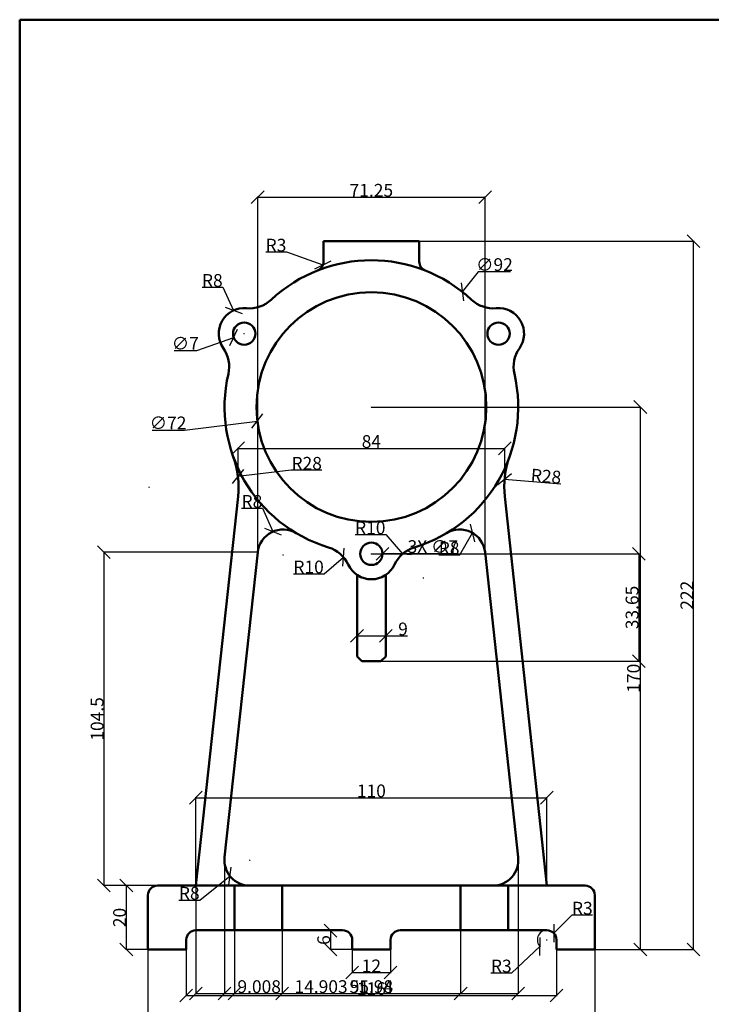
# Model space of a CAD drawing. Units: millimetres. Extents: x -13 to 343, y 323 to 787.
# Tile 2 of 3: x -13 to 204, y 479 to 787. Entities that reach past the tile are written whole.
import ezdxf

# ---------------------------------------------------------------- set-up
doc = ezdxf.new("R2010")
doc.units = ezdxf.units.MM
doc.header["$MEASUREMENT"] = 0
doc.header["$PDMODE"] = 3
doc.header["$PDSIZE"] = -8
for name, color, linetype, lineweight in [('M-DIMS', 2, 'Continuous', 25), ('M-OUTL', 7, 'Continuous', 50), ('M-TTLB', 7, 'Continuous', 50)]:
    doc.layers.add(name, color=color, linetype=linetype, lineweight=lineweight)
doc.styles.get("Standard").update_dxf_attribs({"font": 'arial.ttf'})
doc.dimstyles.get("Standard").update_dxf_attribs({"dimtxt": 4, "dimasz": 4, "dimexe": 0.18, "dimexo": 0.0625, "dimgap": 0.09, "dimtad": 1, "dimtoh": 1, "dimdec": 0, "dimzin": 0, "dimdsep": 46, "dimtxsty": 'Standard', "dimblk": 'OBLIQUE', "dimcen": 0.09, "dimclre": 251, "dimadec": 0, "dimazin": 0, "dimtfac": 1, "dimtdec": 0, "dimtofl": 0, "dimtmove": 0, "dimatfit": 3, "dimfxl": 1, "dimtolj": 1, "dimtzin": 0, "dimarcsym": 0})

# ---------------------------------------------------------------- blocks, each defined once
blk = doc.blocks.new('_Oblique')
at = {"color": 0, "linetype": 'ByBlock', "lineweight": -2}
blk.add_line((-0.5, -0.5), (0.5, 0.5), dxfattribs=at)
blk = doc.blocks.new('*D4')
at = {"layer": 'Defpoints', "color": 0, "transparency": 16777216}
for p in [(79.05, 711.47), (81.88, 710.47)]:
    blk.add_point(p, dxfattribs=at)
at = {"layer": 'M-DIMS', "color": 0, "lineweight": -2, "transparency": 16777216}
for p, q in [((63.95, 714.5), (70.49, 714.5)), ((70.49, 714.5), (81.88, 710.47))]:
    blk.add_line(p, q, dxfattribs=at)
at = {"layer": 'M-DIMS', "color": 0, "lineweight": -2, "transparency": 16777216, "xscale": 4, "yscale": 4, "zscale": 4, "rotation": 340.5270961751787}
blk.add_blockref('_Oblique', (81.88, 710.47), dxfattribs=at)
at = {"layer": 'M-DIMS', "color": 0, "transparency": 16777216, "insert": (67.17, 716.63), "char_height": 4, "attachment_point": 5}
blk.add_mtext('\\A1;R3', dxfattribs=at)
blk = doc.blocks.new('*D5')
at = {"layer": 'Defpoints', "color": 0, "transparency": 16777216}
for p in [(53.88, 696.17), (57.22, 688.9)]:
    blk.add_point(p, dxfattribs=at)
at = {"layer": 'M-DIMS', "color": 0, "lineweight": -2, "transparency": 16777216}
for p, q in [((43.99, 703.43), (50.54, 703.43)), ((50.54, 703.43), (53.88, 696.17)), ((57.13, 688.9), (57.31, 688.9)), ((57.22, 688.81), (57.22, 688.99))]:
    blk.add_line(p, q, dxfattribs=at)
at = {"layer": 'M-DIMS', "color": 0, "lineweight": -2, "transparency": 16777216, "xscale": 4, "yscale": 4, "zscale": 4, "rotation": 294.6792634870832}
blk.add_blockref('_Oblique', (53.88, 696.17), dxfattribs=at)
at = {"layer": 'M-DIMS', "color": 0, "transparency": 16777216, "insert": (47.22, 705.57), "char_height": 4, "attachment_point": 5}
blk.add_mtext('\\A1;R8', dxfattribs=at)
blk = doc.blocks.new('*D6')
at = {"layer": 'Defpoints', "color": 0, "transparency": 16777216}
for p in [(138.77, 643.18), (166.67, 640.82)]:
    blk.add_point(p, dxfattribs=at)
at = {"layer": 'M-DIMS', "color": 0, "lineweight": -2, "transparency": 16777216}
blk.add_line((156.46, 641.69), (138.77, 643.18), dxfattribs=at)
at = {"layer": 'M-DIMS', "color": 0, "lineweight": -2, "transparency": 16777216, "xscale": 4, "yscale": 4, "zscale": 4, "rotation": 175.1553930412952}
blk.add_blockref('_Oblique', (138.77, 643.18), dxfattribs=at)
at = {"layer": 'M-DIMS', "color": 0, "transparency": 16777216, "insert": (151.78, 644.22), "char_height": 4, "attachment_point": 5, "rotation": 355.1554}
blk.add_mtext('\\A1;R28', dxfattribs=at)
blk = doc.blocks.new('*D7')
at = {"layer": 'Defpoints', "color": 0, "transparency": 16777216}
for p in [(88.31, 618.84), (80.72, 612.33)]:
    blk.add_point(p, dxfattribs=at)
at = {"layer": 'M-DIMS', "color": 0, "lineweight": -2, "transparency": 16777216}
for p, q in [((82.24, 613.63), (88.31, 618.84)), ((72.6, 613.63), (82.24, 613.63))]:
    blk.add_line(p, q, dxfattribs=at)
at = {"layer": 'M-DIMS', "color": 0, "lineweight": -2, "transparency": 16777216, "xscale": 4, "yscale": 4, "zscale": 4, "rotation": 40.60279433407489}
blk.add_blockref('_Oblique', (88.31, 618.84), dxfattribs=at)
at = {"layer": 'M-DIMS', "color": 0, "transparency": 16777216, "insert": (77.38, 615.76), "char_height": 4, "attachment_point": 5}
blk.add_mtext('\\A1;R10', dxfattribs=at)
blk = doc.blocks.new('*D8')
at = {"layer": 'Defpoints', "color": 0, "transparency": 16777216}
for p in [(128.77, 626.43), (124.73, 619.53)]:
    blk.add_point(p, dxfattribs=at)
at = {"layer": 'M-DIMS', "color": 0, "lineweight": -2, "transparency": 16777216}
for p, q in [((124.73, 619.53), (128.77, 626.43)), ((118.18, 619.53), (124.73, 619.53))]:
    blk.add_line(p, q, dxfattribs=at)
at = {"layer": 'M-DIMS', "color": 0, "lineweight": -2, "transparency": 16777216, "xscale": 4, "yscale": 4, "zscale": 4, "rotation": 59.62070806572377}
blk.add_blockref('_Oblique', (128.77, 626.43), dxfattribs=at)
at = {"layer": 'M-DIMS', "color": 0, "transparency": 16777216, "insert": (121.41, 621.66), "char_height": 4, "attachment_point": 5}
blk.add_mtext('\\A1;R8', dxfattribs=at)
blk = doc.blocks.new('*D9')
at = {"layer": 'Defpoints', "color": 0, "transparency": 16777216}
for p in [(152.05, 498.9), (149.87, 496.84)]:
    blk.add_point(p, dxfattribs=at)
at = {"layer": 'M-DIMS', "color": 0, "lineweight": -2, "transparency": 16777216}
for p, q in [((151.96, 498.9), (152.14, 498.9)), ((152.05, 498.81), (152.05, 498.99)), ((141.07, 488.55), (149.87, 496.84)), ((134.53, 488.55), (141.07, 488.55))]:
    blk.add_line(p, q, dxfattribs=at)
blk.add_arc((152.05, 498.9), 3, 91.1937, 226.7257, dxfattribs=at)
at = {"layer": 'M-DIMS', "color": 0, "lineweight": -2, "transparency": 16777216, "xscale": 4, "yscale": 4, "zscale": 4, "rotation": 43.28792637846206}
blk.add_blockref('_Oblique', (149.87, 496.84), dxfattribs=at)
at = {"layer": 'M-DIMS', "color": 0, "transparency": 16777216, "insert": (137.76, 490.68), "char_height": 4, "attachment_point": 5}
blk.add_mtext('\\A1;R3', dxfattribs=at)
blk = doc.blocks.new('*D10')
at = {"layer": 'Defpoints', "color": 0, "transparency": 16777216}
for p in [(125.54, 702.01), (68.56, 629.78)]:
    blk.add_point(p, dxfattribs=at)
at = {"layer": 'M-DIMS', "color": 0, "lineweight": -2, "transparency": 16777216}
for p, q in [((130.5, 708.29), (125.54, 702.01)), ((140.63, 708.29), (130.5, 708.29)), ((96.96, 665.9), (97.14, 665.9)), ((97.05, 665.81), (97.05, 665.99))]:
    blk.add_line(p, q, dxfattribs=at)
at = {"layer": 'M-DIMS', "color": 0, "lineweight": -2, "transparency": 16777216, "xscale": 4, "yscale": 4, "zscale": 4, "rotation": 231.7324011261606}
blk.add_blockref('_Oblique', (125.54, 702.01), dxfattribs=at)
at = {"layer": 'M-DIMS', "color": 0, "transparency": 16777216, "insert": (135.61, 710.54), "char_height": 4, "attachment_point": 5}
blk.add_mtext('\\A1;∅92', dxfattribs=at)
blk = doc.blocks.new('*D11')
at = {"layer": 'Defpoints', "color": 0, "transparency": 16777216}
for p in [(132.78, 670.3), (61.32, 661.49)]:
    blk.add_point(p, dxfattribs=at)
at = {"layer": 'M-DIMS', "color": 0, "lineweight": -2, "transparency": 16777216}
for p, q in [((96.96, 665.9), (97.14, 665.9)), ((97.05, 665.81), (97.05, 665.99)), ((38.45, 658.68), (61.32, 661.49)), ((28.32, 658.68), (38.45, 658.68))]:
    blk.add_line(p, q, dxfattribs=at)
at = {"layer": 'M-DIMS', "color": 0, "lineweight": -2, "transparency": 16777216, "xscale": 4, "yscale": 4, "zscale": 4, "rotation": 7.023598730046072}
blk.add_blockref('_Oblique', (61.32, 661.49), dxfattribs=at)
at = {"layer": 'M-DIMS', "color": 0, "transparency": 16777216, "insert": (33.34, 660.92), "char_height": 4, "attachment_point": 5}
blk.add_mtext('\\A1;∅72', dxfattribs=at)
blk = doc.blocks.new('*D12')
at = {"layer": 'Defpoints', "color": 0, "transparency": 16777216}
for p in [(60.51, 690.07), (53.92, 687.72)]:
    blk.add_point(p, dxfattribs=at)
at = {"layer": 'M-DIMS', "color": 0, "lineweight": -2, "transparency": 16777216}
for p, q in [((57.13, 688.9), (57.31, 688.9)), ((57.22, 688.81), (57.22, 688.99)), ((42.33, 683.58), (53.92, 687.72)), ((35.26, 683.58), (42.33, 683.58))]:
    blk.add_line(p, q, dxfattribs=at)
at = {"layer": 'M-DIMS', "color": 0, "lineweight": -2, "transparency": 16777216, "xscale": 4, "yscale": 4, "zscale": 4, "rotation": 19.63186523037221}
blk.add_blockref('_Oblique', (53.92, 687.72), dxfattribs=at)
at = {"layer": 'M-DIMS', "color": 0, "transparency": 16777216, "insert": (38.75, 685.83), "char_height": 4, "attachment_point": 5}
blk.add_mtext('\\A1;∅7', dxfattribs=at)
blk = doc.blocks.new('*D13')
at = {"layer": 'Defpoints', "color": 0, "transparency": 16777216}
for p in [(97.14, 665.9), (167.05, 495.9), (181.31, 495.9)]:
    blk.add_point(p, dxfattribs=at)
at = {"layer": 'M-DIMS', "color": 0, "lineweight": -2, "transparency": 16777216}
for p, q in [((97.21, 665.9), (181.49, 665.9)), ((181.31, 665.9), (181.31, 495.9)), ((167.12, 495.9), (181.49, 495.9))]:
    blk.add_line(p, q, dxfattribs=at)
at = {"layer": 'M-DIMS', "color": 0, "lineweight": -2, "transparency": 16777216, "xscale": 4, "yscale": 4, "zscale": 4}
for p, rotation in [((181.31, 665.9), 90), ((181.31, 495.9), 270)]:
    blk.add_blockref('_Oblique', p, dxfattribs=dict(at, rotation=rotation))
at = {"layer": 'M-DIMS', "color": 0, "transparency": 16777216, "insert": (179.18, 580.9), "char_height": 4, "attachment_point": 5, "rotation": 90}
blk.add_mtext('\\A1;170', dxfattribs=at)
blk = doc.blocks.new('*D14')
at = {"layer": 'Defpoints', "color": 0, "transparency": 16777216}
for p in [(112.05, 717.9), (198, 717.9), (167.05, 495.9)]:
    blk.add_point(p, dxfattribs=at)
at = {"layer": 'M-DIMS', "color": 0, "lineweight": -2, "transparency": 16777216}
for p, q in [((112.12, 717.9), (198.18, 717.9)), ((198, 495.9), (198, 717.9)), ((167.12, 495.9), (198.18, 495.9))]:
    blk.add_line(p, q, dxfattribs=at)
at = {"layer": 'M-DIMS', "color": 0, "lineweight": -2, "transparency": 16777216, "xscale": 4, "yscale": 4, "zscale": 4}
for p, rotation in [((198, 717.9), 90), ((198, 495.9), 270)]:
    blk.add_blockref('_Oblique', p, dxfattribs=dict(at, rotation=rotation))
at = {"layer": 'M-DIMS', "color": 0, "transparency": 16777216, "insert": (195.9, 606.9), "char_height": 4, "attachment_point": 5, "rotation": 90}
blk.add_mtext('\\A1;222', dxfattribs=at)
blk = doc.blocks.new('*D15')
at = {"layer": 'Defpoints', "color": 0, "transparency": 16777216}
for p in [(27.05, 495.9), (167.05, 495.9), (167.05, 471.86)]:
    blk.add_point(p, dxfattribs=at)
at = {"layer": 'M-DIMS', "color": 0, "lineweight": -2, "transparency": 16777216}
for p, q in [((27.05, 495.83), (27.05, 471.68)), ((167.05, 495.83), (167.05, 471.68)), ((27.05, 471.86), (167.05, 471.86))]:
    blk.add_line(p, q, dxfattribs=at)
at = {"layer": 'M-DIMS', "color": 0, "lineweight": -2, "transparency": 16777216, "xscale": 4, "yscale": 4, "zscale": 4, "rotation": 180}
blk.add_blockref('_Oblique', (27.05, 471.86), dxfattribs=at)
at = {"layer": 'M-DIMS', "color": 0, "lineweight": -2, "transparency": 16777216, "xscale": 4, "yscale": 4, "zscale": 4}
blk.add_blockref('_Oblique', (167.05, 471.86), dxfattribs=at)
at = {"layer": 'M-DIMS', "color": 0, "transparency": 16777216, "insert": (97.05, 473.99), "char_height": 4, "attachment_point": 5}
blk.add_mtext('\\A1;140', dxfattribs=at)
blk = doc.blocks.new('*D16')
at = {"layer": 'Defpoints', "color": 0, "transparency": 16777216}
for p in [(39.05, 495.9), (155.05, 495.9), (155.05, 481.47)]:
    blk.add_point(p, dxfattribs=at)
at = {"layer": 'M-DIMS', "color": 0, "lineweight": -2, "transparency": 16777216}
for p, q in [((39.05, 495.83), (39.05, 481.29)), ((155.05, 495.83), (155.05, 481.29)), ((39.05, 481.47), (155.05, 481.47))]:
    blk.add_line(p, q, dxfattribs=at)
at = {"layer": 'M-DIMS', "color": 0, "lineweight": -2, "transparency": 16777216, "xscale": 4, "yscale": 4, "zscale": 4, "rotation": 180}
blk.add_blockref('_Oblique', (39.05, 481.47), dxfattribs=at)
at = {"layer": 'M-DIMS', "color": 0, "lineweight": -2, "transparency": 16777216, "xscale": 4, "yscale": 4, "zscale": 4}
blk.add_blockref('_Oblique', (155.05, 481.47), dxfattribs=at)
at = {"layer": 'M-DIMS', "color": 0, "transparency": 16777216, "insert": (97.05, 483.6), "char_height": 4, "attachment_point": 5}
blk.add_mtext('\\A1;116', dxfattribs=at)
blk = doc.blocks.new('*D17')
at = {"layer": 'Defpoints', "color": 0, "transparency": 16777216}
for p in [(88.96, 501.76), (84.26, 495.9), (91.05, 495.9)]:
    blk.add_point(p, dxfattribs=at)
at = {"layer": 'M-DIMS', "color": 0, "lineweight": -2, "transparency": 16777216}
for p, q in [((88.9, 501.76), (84.08, 501.76)), ((84.26, 501.76), (84.26, 495.9)), ((90.99, 495.9), (84.08, 495.9))]:
    blk.add_line(p, q, dxfattribs=at)
at = {"layer": 'M-DIMS', "color": 0, "lineweight": -2, "transparency": 16777216, "xscale": 4, "yscale": 4, "zscale": 4}
for p, rotation in [((84.26, 501.76), 90), ((84.26, 495.9), 270)]:
    blk.add_blockref('_Oblique', p, dxfattribs=dict(at, rotation=rotation))
at = {"layer": 'M-DIMS', "color": 0, "transparency": 16777216, "insert": (82.12, 498.83), "char_height": 4, "attachment_point": 5, "rotation": 90}
blk.add_mtext('\\A1;6', dxfattribs=at)
blk = doc.blocks.new('*D18')
at = {"layer": 'Defpoints', "color": 0, "transparency": 16777216}
for p in [(91.05, 495.9), (103.05, 495.9), (103.05, 488.62)]:
    blk.add_point(p, dxfattribs=at)
at = {"layer": 'M-DIMS', "color": 0, "lineweight": -2, "transparency": 16777216}
for p, q in [((91.05, 495.83), (91.05, 488.44)), ((103.05, 495.83), (103.05, 488.44)), ((91.05, 488.62), (103.05, 488.62))]:
    blk.add_line(p, q, dxfattribs=at)
at = {"layer": 'M-DIMS', "color": 0, "lineweight": -2, "transparency": 16777216, "xscale": 4, "yscale": 4, "zscale": 4, "rotation": 180}
blk.add_blockref('_Oblique', (91.05, 488.62), dxfattribs=at)
at = {"layer": 'M-DIMS', "color": 0, "lineweight": -2, "transparency": 16777216, "xscale": 4, "yscale": 4, "zscale": 4}
blk.add_blockref('_Oblique', (103.05, 488.62), dxfattribs=at)
at = {"layer": 'M-DIMS', "color": 0, "transparency": 16777216, "insert": (97.05, 490.72), "char_height": 4, "attachment_point": 5}
blk.add_mtext('\\A1;12', dxfattribs=at)
blk = doc.blocks.new('*D19')
at = {"layer": 'Defpoints', "color": 0, "transparency": 16777216}
for p in [(20.28, 515.9), (33.13, 515.9), (27.05, 495.9)]:
    blk.add_point(p, dxfattribs=at)
at = {"layer": 'M-DIMS', "color": 0, "lineweight": -2, "transparency": 16777216}
for p, q in [((33.07, 515.9), (20.1, 515.9)), ((20.28, 495.9), (20.28, 515.9)), ((26.99, 495.9), (20.1, 495.9))]:
    blk.add_line(p, q, dxfattribs=at)
at = {"layer": 'M-DIMS', "color": 0, "lineweight": -2, "transparency": 16777216, "xscale": 4, "yscale": 4, "zscale": 4}
for p, rotation in [((20.28, 515.9), 90), ((20.28, 495.9), 270)]:
    blk.add_blockref('_Oblique', p, dxfattribs=dict(at, rotation=rotation))
at = {"layer": 'M-DIMS', "color": 0, "transparency": 16777216, "insert": (18.15, 505.9), "char_height": 4, "attachment_point": 5, "rotation": 90}
blk.add_mtext('\\A1;20', dxfattribs=at)
blk = doc.blocks.new('*D20')
at = {"layer": 'Defpoints', "color": 0, "transparency": 16777216}
for p in [(152.05, 543.45), (42.05, 515.9), (152.05, 515.9)]:
    blk.add_point(p, dxfattribs=at)
at = {"layer": 'M-DIMS', "color": 0, "lineweight": -2, "transparency": 16777216}
for p, q in [((42.05, 515.96), (42.05, 543.63)), ((42.05, 543.45), (152.05, 543.45)), ((152.05, 515.96), (152.05, 543.63))]:
    blk.add_line(p, q, dxfattribs=at)
at = {"layer": 'M-DIMS', "color": 0, "lineweight": -2, "transparency": 16777216, "xscale": 4, "yscale": 4, "zscale": 4, "rotation": 180}
blk.add_blockref('_Oblique', (42.05, 543.45), dxfattribs=at)
at = {"layer": 'M-DIMS', "color": 0, "lineweight": -2, "transparency": 16777216, "xscale": 4, "yscale": 4, "zscale": 4}
blk.add_blockref('_Oblique', (152.05, 543.45), dxfattribs=at)
at = {"layer": 'M-DIMS', "color": 0, "transparency": 16777216, "insert": (97.05, 545.58), "char_height": 4, "attachment_point": 5}
blk.add_mtext('\\A1;110', dxfattribs=at)
blk = doc.blocks.new('*D21')
at = {"layer": 'Defpoints', "color": 0, "transparency": 16777216}
for p in [(138.84, 652.95), (55.27, 637.8), (138.84, 637.8)]:
    blk.add_point(p, dxfattribs=at)
at = {"layer": 'M-DIMS', "color": 0, "lineweight": -2, "transparency": 16777216}
for p, q in [((55.27, 637.86), (55.27, 653.13)), ((55.27, 652.95), (138.84, 652.95)), ((138.84, 637.86), (138.84, 653.13))]:
    blk.add_line(p, q, dxfattribs=at)
at = {"layer": 'M-DIMS', "color": 0, "lineweight": -2, "transparency": 16777216, "xscale": 4, "yscale": 4, "zscale": 4, "rotation": 180}
blk.add_blockref('_Oblique', (55.27, 652.95), dxfattribs=at)
at = {"layer": 'M-DIMS', "color": 0, "lineweight": -2, "transparency": 16777216, "xscale": 4, "yscale": 4, "zscale": 4}
blk.add_blockref('_Oblique', (138.84, 652.95), dxfattribs=at)
at = {"layer": 'M-DIMS', "color": 0, "transparency": 16777216, "insert": (97.05, 655.08), "char_height": 4, "attachment_point": 5}
blk.add_mtext('\\A1;84', dxfattribs=at)
blk = doc.blocks.new('*D22')
at = {"layer": 'Defpoints', "color": 0, "transparency": 16777216}
for p in [(101.55, 594.2), (92.55, 591.73), (101.55, 591.73)]:
    blk.add_point(p, dxfattribs=at)
at = {"layer": 'M-DIMS', "color": 0, "lineweight": -2, "transparency": 16777216}
for p, q in [((92.55, 591.79), (92.55, 594.38)), ((92.55, 594.2), (101.55, 594.2)), ((101.55, 591.79), (101.55, 594.38)), ((101.55, 594.2), (108.36, 594.2))]:
    blk.add_line(p, q, dxfattribs=at)
at = {"layer": 'M-DIMS', "color": 0, "lineweight": -2, "transparency": 16777216, "xscale": 4, "yscale": 4, "zscale": 4, "rotation": 180}
blk.add_blockref('_Oblique', (92.55, 594.2), dxfattribs=at)
at = {"layer": 'M-DIMS', "color": 0, "lineweight": -2, "transparency": 16777216, "xscale": 4, "yscale": 4, "zscale": 4}
blk.add_blockref('_Oblique', (101.55, 594.2), dxfattribs=at)
at = {"layer": 'M-DIMS', "color": 0, "transparency": 16777216, "insert": (106.96, 596.33), "char_height": 4, "attachment_point": 5}
blk.add_mtext('\\A1;9', dxfattribs=at)
blk = doc.blocks.new('*D38')
at = {"layer": 'Defpoints', "color": 0, "transparency": 16777216}
for p in [(97.05, 619.9), (94.05, 586.24), (180.85, 586.24)]:
    blk.add_point(p, dxfattribs=at)
at = {"layer": 'M-DIMS', "color": 251, "lineweight": -2, "transparency": 16777216}
for p, q in [((97.12, 619.9), (181.03, 619.9)), ((94.12, 586.24), (181.03, 586.24))]:
    blk.add_line(p, q, dxfattribs=at)
at = {"layer": 'M-DIMS', "color": 0, "lineweight": -2, "transparency": 16777216}
blk.add_line((180.85, 619.9), (180.85, 586.24), dxfattribs=at)
at = {"layer": 'M-DIMS', "color": 0, "lineweight": -2, "transparency": 16777216, "xscale": 4, "yscale": 4, "zscale": 4}
for p, rotation in [((180.85, 619.9), 90), ((180.85, 586.24), 270)]:
    blk.add_blockref('_Oblique', p, dxfattribs=dict(at, rotation=rotation))
at = {"layer": 'M-DIMS', "color": 0, "transparency": 16777216, "insert": (178.72, 603.07), "char_height": 4, "attachment_point": 5, "rotation": 90}
blk.add_mtext('\\A1;33.65', dxfattribs=at)
blk = doc.blocks.new('*D39')
at = {"layer": 'Defpoints', "color": 0, "transparency": 16777216}
for p in [(132.68, 731.7), (61.43, 620.39), (132.68, 620.39)]:
    blk.add_point(p, dxfattribs=at)
at = {"layer": 'M-DIMS', "color": 251, "lineweight": -2, "transparency": 16777216}
for p, q in [((61.43, 620.45), (61.43, 731.88)), ((132.68, 620.45), (132.68, 731.88))]:
    blk.add_line(p, q, dxfattribs=at)
at = {"layer": 'M-DIMS', "color": 0, "lineweight": -2, "transparency": 16777216}
blk.add_line((61.43, 731.7), (132.68, 731.7), dxfattribs=at)
at = {"layer": 'M-DIMS', "color": 0, "lineweight": -2, "transparency": 16777216, "xscale": 4, "yscale": 4, "zscale": 4, "rotation": 180}
blk.add_blockref('_Oblique', (61.43, 731.7), dxfattribs=at)
at = {"layer": 'M-DIMS', "color": 0, "lineweight": -2, "transparency": 16777216, "xscale": 4, "yscale": 4, "zscale": 4}
blk.add_blockref('_Oblique', (132.68, 731.7), dxfattribs=at)
at = {"layer": 'M-DIMS', "color": 0, "transparency": 16777216, "insert": (97.05, 733.83), "char_height": 4, "attachment_point": 5}
blk.add_mtext('\\A1;71.25', dxfattribs=at)
blk = doc.blocks.new('*D40')
at = {"layer": 'Defpoints', "color": 0, "transparency": 16777216}
for p in [(51.06, 524.76), (143.05, 524.76), (143.05, 482.1)]:
    blk.add_point(p, dxfattribs=at)
at = {"layer": 'M-DIMS', "color": 251, "lineweight": -2, "transparency": 16777216}
for p, q in [((51.06, 524.7), (51.06, 481.92)), ((143.05, 524.7), (143.05, 481.92))]:
    blk.add_line(p, q, dxfattribs=at)
at = {"layer": 'M-DIMS', "color": 0, "lineweight": -2, "transparency": 16777216}
blk.add_line((51.06, 482.1), (143.05, 482.1), dxfattribs=at)
at = {"layer": 'M-DIMS', "color": 0, "lineweight": -2, "transparency": 16777216, "xscale": 4, "yscale": 4, "zscale": 4, "rotation": 180}
blk.add_blockref('_Oblique', (51.06, 482.1), dxfattribs=at)
at = {"layer": 'M-DIMS', "color": 0, "lineweight": -2, "transparency": 16777216, "xscale": 4, "yscale": 4, "zscale": 4}
blk.add_blockref('_Oblique', (143.05, 482.1), dxfattribs=at)
at = {"layer": 'M-DIMS', "color": 0, "transparency": 16777216, "insert": (97.05, 484.23), "char_height": 4, "attachment_point": 5}
blk.add_mtext('\\A1;91.98', dxfattribs=at)
blk = doc.blocks.new('*D41')
at = {"layer": 'Defpoints', "color": 0, "transparency": 16777216}
for p in [(51.06, 524.76), (42.05, 515.9), (51.06, 482.1)]:
    blk.add_point(p, dxfattribs=at)
at = {"layer": 'M-DIMS', "color": 251, "lineweight": -2, "transparency": 16777216}
for p, q in [((51.06, 524.7), (51.06, 481.92)), ((42.05, 515.83), (42.05, 481.92))]:
    blk.add_line(p, q, dxfattribs=at)
at = {"layer": 'M-DIMS', "color": 0, "lineweight": -2, "transparency": 16777216}
for p, q in [((42.05, 482.1), (51.06, 482.1)), ((51.06, 482.1), (68.75, 482.1))]:
    blk.add_line(p, q, dxfattribs=at)
at = {"layer": 'M-DIMS', "color": 0, "lineweight": -2, "transparency": 16777216, "xscale": 4, "yscale": 4, "zscale": 4, "rotation": 180}
blk.add_blockref('_Oblique', (42.05, 482.1), dxfattribs=at)
at = {"layer": 'M-DIMS', "color": 0, "lineweight": -2, "transparency": 16777216, "xscale": 4, "yscale": 4, "zscale": 4}
blk.add_blockref('_Oblique', (51.06, 482.1), dxfattribs=at)
at = {"layer": 'M-DIMS', "color": 0, "transparency": 16777216, "insert": (61.9, 484.23), "char_height": 4, "attachment_point": 5}
blk.add_mtext('\\A1;9.008', dxfattribs=at)
blk = doc.blocks.new('*D42')
at = {"layer": 'Defpoints', "color": 0, "transparency": 16777216}
for p in [(61.43, 620.39), (13.25, 515.9), (59.01, 515.9)]:
    blk.add_point(p, dxfattribs=at)
at = {"layer": 'M-DIMS', "color": 251, "lineweight": -2, "transparency": 16777216}
for p, q in [((61.36, 620.39), (13.07, 620.39)), ((58.95, 515.9), (13.07, 515.9))]:
    blk.add_line(p, q, dxfattribs=at)
at = {"layer": 'M-DIMS', "color": 0, "lineweight": -2, "transparency": 16777216}
blk.add_line((13.25, 620.39), (13.25, 515.9), dxfattribs=at)
at = {"layer": 'M-DIMS', "color": 0, "lineweight": -2, "transparency": 16777216, "xscale": 4, "yscale": 4, "zscale": 4}
for p, rotation in [((13.25, 620.39), 90), ((13.25, 515.9), 270)]:
    blk.add_blockref('_Oblique', p, dxfattribs=dict(at, rotation=rotation))
at = {"layer": 'M-DIMS', "color": 0, "transparency": 16777216, "insert": (11.12, 568.14), "char_height": 4, "attachment_point": 5, "rotation": 90}
blk.add_mtext('\\A1;104.5', dxfattribs=at)
blk = doc.blocks.new('*D43')
at = {"layer": 'Defpoints', "color": 0, "transparency": 16777216}
for p in [(54.18, 515.9), (69.08, 515.9), (69.08, 482.1)]:
    blk.add_point(p, dxfattribs=at)
at = {"layer": 'M-DIMS', "color": 251, "lineweight": -2, "transparency": 16777216}
for p, q in [((54.18, 515.83), (54.18, 481.92)), ((69.08, 515.83), (69.08, 481.92))]:
    blk.add_line(p, q, dxfattribs=at)
at = {"layer": 'M-DIMS', "color": 0, "lineweight": -2, "transparency": 16777216}
for p, q in [((54.18, 482.1), (69.08, 482.1)), ((69.08, 482.1), (89.49, 482.1))]:
    blk.add_line(p, q, dxfattribs=at)
at = {"layer": 'M-DIMS', "color": 0, "lineweight": -2, "transparency": 16777216, "xscale": 4, "yscale": 4, "zscale": 4, "rotation": 180}
blk.add_blockref('_Oblique', (54.18, 482.1), dxfattribs=at)
at = {"layer": 'M-DIMS', "color": 0, "lineweight": -2, "transparency": 16777216, "xscale": 4, "yscale": 4, "zscale": 4}
blk.add_blockref('_Oblique', (69.08, 482.1), dxfattribs=at)
at = {"layer": 'M-DIMS', "color": 0, "transparency": 16777216, "insert": (81.29, 484.23), "char_height": 4, "attachment_point": 5}
blk.add_mtext('\\A1;14.903', dxfattribs=at)
blk = doc.blocks.new('*D44')
at = {"layer": 'Defpoints', "color": 0, "transparency": 16777216}
for p in [(69.08, 515.9), (125.02, 515.9), (125.02, 482.1)]:
    blk.add_point(p, dxfattribs=at)
at = {"layer": 'M-DIMS', "color": 251, "lineweight": -2, "transparency": 16777216}
for p, q in [((69.08, 515.83), (69.08, 481.92)), ((125.02, 515.83), (125.02, 481.92))]:
    blk.add_line(p, q, dxfattribs=at)
at = {"layer": 'M-DIMS', "color": 0, "lineweight": -2, "transparency": 16777216}
blk.add_line((69.08, 482.1), (125.02, 482.1), dxfattribs=at)
at = {"layer": 'M-DIMS', "color": 0, "lineweight": -2, "transparency": 16777216, "xscale": 4, "yscale": 4, "zscale": 4, "rotation": 180}
blk.add_blockref('_Oblique', (69.08, 482.1), dxfattribs=at)
at = {"layer": 'M-DIMS', "color": 0, "lineweight": -2, "transparency": 16777216, "xscale": 4, "yscale": 4, "zscale": 4}
blk.add_blockref('_Oblique', (125.02, 482.1), dxfattribs=at)
at = {"layer": 'M-DIMS', "color": 0, "transparency": 16777216, "insert": (97.05, 484.23), "char_height": 4, "attachment_point": 5}
blk.add_mtext('\\A1;55.94', dxfattribs=at)
blk = doc.blocks.new('*D65')
at = {"layer": 'Defpoints', "color": 0, "transparency": 16777216}
for p in [(93.55, 619.89), (100.55, 619.9)]:
    blk.add_point(p, dxfattribs=at)
at = {"layer": 'M-DIMS', "color": 251, "lineweight": -2, "transparency": 16777216}
for p, q in [((96.96, 619.9), (97.14, 619.9)), ((97.05, 619.81), (97.05, 619.99))]:
    blk.add_line(p, q, dxfattribs=at)
at = {"layer": 'M-DIMS', "color": 0, "lineweight": -2, "transparency": 16777216}
for p, q in [((108.55, 619.91), (100.55, 619.9)), ((124, 619.91), (108.55, 619.91))]:
    blk.add_line(p, q, dxfattribs=at)
at = {"layer": 'M-DIMS', "color": 0, "lineweight": -2, "transparency": 16777216, "xscale": 4, "yscale": 4, "zscale": 4, "rotation": 180.0631563297542}
blk.add_blockref('_Oblique', (100.55, 619.9), dxfattribs=at)
at = {"layer": 'M-DIMS', "color": 0, "transparency": 16777216, "insert": (116.32, 622.15), "char_height": 4, "attachment_point": 5}
blk.add_mtext('\\A1;3X ∅7', dxfattribs=at)
blk = doc.blocks.new('*D66')
at = {"layer": 'Defpoints', "color": 0, "transparency": 16777216}
for p in [(55.23, 644.14), (27.43, 640.82)]:
    blk.add_point(p, dxfattribs=at)
at = {"layer": 'M-DIMS', "color": 0, "lineweight": -2, "transparency": 16777216}
for p, q in [((71.92, 646.13), (55.23, 644.14)), ((81.57, 646.13), (71.92, 646.13))]:
    blk.add_line(p, q, dxfattribs=at)
at = {"layer": 'M-DIMS', "color": 251, "lineweight": -2, "transparency": 16777216}
for p, q in [((27.34, 640.82), (27.52, 640.82)), ((27.43, 640.73), (27.43, 640.91))]:
    blk.add_line(p, q, dxfattribs=at)
at = {"layer": 'M-DIMS', "color": 0, "lineweight": -2, "transparency": 16777216, "xscale": 4, "yscale": 4, "zscale": 4, "rotation": 186.8108270128715}
blk.add_blockref('_Oblique', (55.23, 644.14), dxfattribs=at)
at = {"layer": 'M-DIMS', "color": 0, "transparency": 16777216, "insert": (76.79, 648.26), "char_height": 4, "attachment_point": 5}
blk.add_mtext('\\A1;R28', dxfattribs=at)
blk = doc.blocks.new('*D67')
at = {"layer": 'Defpoints', "color": 0, "transparency": 16777216}
for p in [(106.82, 619.87), (113.39, 612.33)]:
    blk.add_point(p, dxfattribs=at)
at = {"layer": 'M-DIMS', "color": 0, "lineweight": -2, "transparency": 16777216}
for p, q in [((91.93, 625.91), (101.57, 625.91)), ((101.57, 625.91), (106.82, 619.87))]:
    blk.add_line(p, q, dxfattribs=at)
at = {"layer": 'M-DIMS', "color": 251, "lineweight": -2, "transparency": 16777216}
for p, q in [((113.3, 612.33), (113.48, 612.33)), ((113.39, 612.24), (113.39, 612.42))]:
    blk.add_line(p, q, dxfattribs=at)
at = {"layer": 'M-DIMS', "color": 0, "lineweight": -2, "transparency": 16777216, "xscale": 4, "yscale": 4, "zscale": 4, "rotation": 311.0503202395105}
blk.add_blockref('_Oblique', (106.82, 619.87), dxfattribs=at)
at = {"layer": 'M-DIMS', "color": 0, "transparency": 16777216, "insert": (96.7, 628.04), "char_height": 4, "attachment_point": 5}
blk.add_mtext('\\A1;R10', dxfattribs=at)
blk = doc.blocks.new('*D68')
at = {"layer": 'Defpoints', "color": 0, "transparency": 16777216}
for p in [(154.17, 501.02), (152.05, 498.9)]:
    blk.add_point(p, dxfattribs=at)
at = {"layer": 'M-DIMS', "color": 0, "lineweight": -2, "transparency": 16777216}
for p, q in [((159.83, 506.67), (154.17, 501.02)), ((166.37, 506.67), (159.83, 506.67))]:
    blk.add_line(p, q, dxfattribs=at)
at = {"layer": 'M-DIMS', "color": 251, "lineweight": -2, "transparency": 16777216}
for p, q in [((151.96, 498.9), (152.14, 498.9)), ((152.05, 498.81), (152.05, 498.99))]:
    blk.add_line(p, q, dxfattribs=at)
at = {"layer": 'M-DIMS', "color": 0, "lineweight": -2, "transparency": 16777216, "xscale": 4, "yscale": 4, "zscale": 4, "rotation": 225.0000135047453}
blk.add_blockref('_Oblique', (154.17, 501.02), dxfattribs=at)
at = {"layer": 'M-DIMS', "color": 0, "transparency": 16777216, "insert": (163.15, 508.81), "char_height": 4, "attachment_point": 5}
blk.add_mtext('\\A1;R3', dxfattribs=at)
blk = doc.blocks.new('*D69')
at = {"layer": 'Defpoints', "color": 0, "transparency": 16777216}
for p in [(66.17, 626.85), (69.38, 619.53)]:
    blk.add_point(p, dxfattribs=at)
at = {"layer": 'M-DIMS', "color": 0, "lineweight": -2, "transparency": 16777216}
for p, q in [((56.4, 634.18), (62.95, 634.18)), ((62.95, 634.18), (66.17, 626.85))]:
    blk.add_line(p, q, dxfattribs=at)
at = {"layer": 'M-DIMS', "color": 251, "lineweight": -2, "transparency": 16777216}
for p, q in [((69.29, 619.53), (69.47, 619.53)), ((69.38, 619.44), (69.38, 619.62))]:
    blk.add_line(p, q, dxfattribs=at)
at = {"layer": 'M-DIMS', "color": 0, "lineweight": -2, "transparency": 16777216, "xscale": 4, "yscale": 4, "zscale": 4, "rotation": 293.6978424292121}
blk.add_blockref('_Oblique', (66.17, 626.85), dxfattribs=at)
at = {"layer": 'M-DIMS', "color": 0, "transparency": 16777216, "insert": (59.63, 636.31), "char_height": 4, "attachment_point": 5}
blk.add_mtext('\\A1;R8', dxfattribs=at)
blk = doc.blocks.new('*D70')
at = {"layer": 'Defpoints', "color": 0, "transparency": 16777216}
for p in [(59.01, 523.9), (52.76, 518.91)]:
    blk.add_point(p, dxfattribs=at)
at = {"layer": 'M-DIMS', "color": 251, "lineweight": -2, "transparency": 16777216}
for p, q in [((58.92, 523.9), (59.1, 523.9)), ((59.01, 523.81), (59.01, 523.99))]:
    blk.add_line(p, q, dxfattribs=at)
at = {"layer": 'M-DIMS', "color": 0, "lineweight": -2, "transparency": 16777216}
for p, q in [((43.31, 511.38), (52.76, 518.91)), ((36.76, 511.38), (43.31, 511.38))]:
    blk.add_line(p, q, dxfattribs=at)
at = {"layer": 'M-DIMS', "color": 0, "lineweight": -2, "transparency": 16777216, "xscale": 4, "yscale": 4, "zscale": 4, "rotation": 38.5432983527568}
blk.add_blockref('_Oblique', (52.76, 518.91), dxfattribs=at)
at = {"layer": 'M-DIMS', "color": 0, "transparency": 16777216, "insert": (39.99, 513.51), "char_height": 4, "attachment_point": 5}
blk.add_mtext('\\A1;R8', dxfattribs=at)

msp = doc.modelspace()

# ---------------------------------------------------------------- linework, layer by layer
at = {"layer": 'M-OUTL'}
for p, q in [((82.053, 711.4703), (82.053, 717.8961)), ((82.053, 717.8961), (112.053, 717.8961)), ((112.053, 717.8961), (112.053, 711.4703)), ((55.2683, 637.8017), (42.053, 515.8961)), ((152.053, 515.8961), (138.8376, 637.8017)), ((61.4274, 620.3875), (51.0606, 524.7583)), ((143.0454, 524.7583), (132.6785, 620.3875)), ((92.553, 587.7442), (92.553, 613.2818)), ((101.553, 587.7442), (101.553, 613.2818)), ((92.553, 587.7442), (94.053, 586.2442)), ((101.553, 587.7442), (100.053, 586.2442)), ((94.053, 586.2442), (100.053, 586.2442)), ((30.053, 515.8961), (164.053, 515.8961)), ((54.1784, 515.8961), (54.1784, 501.8961)), ((69.0816, 515.8961), (69.0816, 501.8961)), ((125.0243, 515.8961), (125.0243, 501.8961)), ((139.9275, 515.8961), (139.9275, 501.8961)), ((27.053, 495.8961), (27.053, 512.8961)), ((167.053, 512.8961), (167.053, 495.8961)), ((42.053, 501.8961), (88.053, 501.8961)), ((106.053, 501.8961), (152.053, 501.8961)), ((39.053, 495.8961), (39.053, 498.8961)), ((91.053, 498.8961), (91.053, 495.8961)), ((103.053, 498.8961), (103.053, 495.8961)), ((155.053, 498.8961), (155.053, 495.8961)), ((27.053, 495.8961), (39.053, 495.8961)), ((91.053, 495.8961), (103.053, 495.8961)), ((155.053, 495.8961), (167.053, 495.8961))]:
    msp.add_line(p, q, dxfattribs=at)
for centre, radius in [((97.053, 665.8961), 36), ((57.2158, 688.8961), 3.5), ((136.8901, 688.8961), 3.5), ((97.053, 619.8961), 3.5)]:
    msp.add_circle(centre, radius, dxfattribs=at)
for centre, radius, start, end in [((97.053, 665.8961), 46, 46.957426, 133.042574), ((79.053, 711.4703), 3, 291.552089, 0), ((115.053, 711.4703), 3, 180, 248.447911), ((58.8306, 706.8236), 10, 264.852889, 313.042574), ((135.2753, 706.8236), 10, 226.957426, 275.147111), ((57.2158, 688.8961), 8, 84.852889, 215.147111), ((136.8901, 688.8961), 8, 324.852889, 95.147111), ((42.4976, 678.5339), 10, 346.957426, 35.147111), ((151.6083, 678.5339), 10, 144.852889, 193.042574), ((97.053, 665.8961), 46, 166.957426, 253.042574), ((97.053, 665.8961), 46, 286.957426, 13.042574), ((27.4314, 640.8194), 28, 353.812917, 19.80833), ((166.6745, 640.8194), 28, 160.19167, 186.187083), ((69.3808, 619.5253), 8, 59.173009, 173.812917), ((124.7251, 619.5253), 8, 6.187083, 120.826991), ((80.72, 612.3309), 10, 24.852889, 73.042574), ((113.386, 612.3309), 10, 106.957426, 155.147111), ((97.053, 619.8961), 8, 204.852889, 335.147111), ((59.014, 523.8961), 8, 173.812917, 270), ((135.092, 523.8961), 8, 270, 6.187083), ((30.053, 512.8961), 3, 90, 180), ((164.053, 512.8961), 3, 0, 90), ((42.053, 498.8961), 3, 90, 180), ((88.053, 498.8961), 3, 0, 90), ((106.053, 498.8961), 3, 90, 180), ((152.053, 498.8961), 3, 0, 90)]:
    msp.add_arc(centre, radius, start, end, dxfattribs=at)
at = {"layer": 'M-TTLB'}
msp.add_lwpolyline([(-13.1348, 787.3025), (332.5007, 787.3025), (332.5007, 323.2082), (-13.1348, 323.2082)], close=True, dxfattribs=at)

# ---------------------------------------------------------------- dimensions: what is measured, and where the dimension line sits
at = {"layer": 'M-DIMS'}
for base, p1, p2, override, picture, middle in [((132.6785, 731.6961), (61.4274, 620.3875), (132.6785, 620.3875), {"dimdec": 2, "dimlfac": 1, "dimrnd": 0, "dimzin": 0, "dimdsep": 46, "dimlunit": 2}, '*D39', (97.053, 733.8284)), ((138.8376, 652.9461), (55.2683, 637.8017), (138.8376, 637.8017), {"dimclrd": 0, "dimclre": 0, "dimclrt": 0}, '*D21', (97.053, 655.0784)), ((152.053, 543.4516), (42.053, 515.8961), (152.053, 515.8961), {"dimclrd": 0, "dimclre": 0, "dimclrt": 0}, '*D20', (97.053, 545.5839)), ((51.0606, 482.0961), (42.053, 515.8961), (51.0606, 524.7583), {"dimdec": 3, "dimlfac": 1, "dimrnd": 0, "dimzin": 0, "dimdsep": 46, "dimlunit": 2}, '*D41', (61.9036, 484.2284)), ((143.0454, 482.0961), (51.0606, 524.7583), (143.0454, 524.7583), {"dimdec": 2, "dimlfac": 1, "dimrnd": 0, "dimzin": 0, "dimdsep": 46, "dimlunit": 2}, '*D40', (97.053, 484.2284)), ((69.0816, 482.0961), (54.1784, 515.8961), (69.0816, 515.8961), {"dimdec": 3, "dimlfac": 1, "dimrnd": 0, "dimzin": 0, "dimdsep": 46, "dimlunit": 2}, '*D43', (81.2862, 484.2298)), ((125.0243, 482.0961), (69.0816, 515.8961), (125.0243, 515.8961), {"dimdec": 2, "dimlfac": 1, "dimrnd": 0, "dimzin": 0, "dimdsep": 46, "dimlunit": 2}, '*D44', (97.053, 484.2284)), ((167.053, 471.8556), (27.053, 495.8961), (167.053, 495.8961), {"dimclrd": 0, "dimclre": 0, "dimclrt": 0}, '*D15', (97.053, 473.9879)), ((155.053, 481.4679), (39.053, 495.8961), (155.053, 495.8961), {"dimclrd": 0, "dimclre": 0, "dimclrt": 0}, '*D16', (97.053, 483.6002)), ((103.053, 488.6207), (91.053, 495.8961), (103.053, 495.8961), {"dimclrd": 0, "dimclre": 0, "dimclrt": 0}, '*D18', (97.053, 490.7189))]:
    dim = msp.add_linear_dim(base=base, p1=p1, p2=p2, dimstyle='Standard', override=override, dxfattribs=at)
    dim.commit()
    dim.dimension.update_dxf_attribs({"geometry": picture, "text_midpoint": middle})
for center, mpoint, override, picture, middle in [((79.053, 711.4703), (81.8814, 710.4702), {"dimclrd": 0, "dimclre": 0, "dimclrt": 0}, '*D4', (67.1704, 714.4996)), ((27.4314, 640.8194), (55.2338, 644.14), {"dimdec": 0, "dimlfac": 1, "dimrnd": 0, "dimzin": 0, "dimdsep": 46, "dimlunit": 2}, '*D66', (71.9153, 646.1323)), ((166.6745, 640.8194), (138.7745, 643.1841), {"dimclrd": 0, "dimclre": 0, "dimclrt": 0}, '*D6', (151.6016, 642.0969)), ((124.7251, 619.5253), (128.7709, 626.4269), {"dimclrd": 0, "dimclre": 0, "dimclrt": 0}, '*D8', (121.4059, 619.5253)), ((80.72, 612.3309), (88.3124, 618.839), {"dimclrd": 0, "dimclre": 0, "dimclrt": 0}, '*D7', (77.3763, 613.6326))]:
    dim = msp.add_radius_dim(center=center, mpoint=mpoint, dimstyle='Standard', override=override, dxfattribs=at)
    dim.commit()
    dim.dimension.update_dxf_attribs({"geometry": picture, "text_midpoint": middle, "dimtype": 164})
for base, p1, p2, override, picture, middle in [((197.9964, 717.8961), (167.053, 495.8961), (112.053, 717.8961), {"dimclrd": 0, "dimclre": 0, "dimclrt": 0}, '*D14', (195.8982, 606.8961)), ((181.3116, 495.8961), (97.143, 665.8961), (167.053, 495.8961), {"dimclrd": 0, "dimclre": 0, "dimclrt": 0}, '*D13', (179.1793, 580.8961)), ((13.253, 515.8961), (61.4274, 620.3875), (59.014, 515.8961), {"dimdec": 1, "dimlfac": 1, "dimrnd": 0, "dimzin": 0, "dimdsep": 46, "dimlunit": 2}, '*D42', (11.1207, 568.1418)), ((180.853, 586.2442), (97.053, 619.8961), (94.053, 586.2442), {"dimdec": 2, "dimlfac": 1, "dimrnd": 0, "dimzin": 0, "dimdsep": 46, "dimlunit": 2}, '*D38', (178.7193, 603.0702)), ((20.2777, 515.8961), (27.053, 495.8961), (33.1337, 515.8961), {"dimclrd": 0, "dimclre": 0, "dimclrt": 0}, '*D19', (18.1454, 505.8961)), ((84.2553, 495.8961), (88.9603, 501.7557), (91.053, 495.8961), {"dimclrd": 0, "dimclre": 0, "dimclrt": 0}, '*D17', (82.123, 498.8259))]:
    dim = msp.add_linear_dim(base=base, p1=p1, p2=p2, angle=90, dimstyle='Standard', override=override, dxfattribs=at)
    dim.commit()
    dim.dimension.update_dxf_attribs({"geometry": picture, "text_midpoint": middle})
for p1, p2, picture, middle in [((68.5636, 629.7803), (125.5424, 702.012), '*D10', (135.6075, 710.5371)), ((60.5124, 690.0721), (53.9193, 687.7202), '*D12', (38.7494, 685.8291))]:
    dim = msp.add_diameter_dim_2p(p1=p1, p2=p2, dimstyle='Standard', override={"dimclrd": 0, "dimclre": 0, "dimclrt": 0}, dxfattribs=at)
    dim.commit()
    dim.dimension.update_dxf_attribs({"geometry": picture, "text_midpoint": middle})
for center, mpoint, override, picture, middle in [((57.2158, 688.8961), (53.8755, 696.1654), {"dimclrd": 0, "dimclre": 0, "dimclrt": 0}, '*D5', (47.216, 705.567)), ((69.3808, 619.5253), (66.1655, 626.8508), {"dimdec": 0, "dimlfac": 1, "dimrnd": 0, "dimzin": 0, "dimdsep": 46, "dimlunit": 2}, '*D69', (59.631, 636.3085)), ((113.386, 612.3309), (106.8188, 619.8723), {"dimdec": 0, "dimlfac": 1, "dimrnd": 0, "dimzin": 0, "dimdsep": 46, "dimlunit": 2}, '*D67', (96.7028, 628.0376)), ((59.014, 523.8961), (52.7569, 518.9113), {"dimdec": 0, "dimlfac": 1, "dimrnd": 0, "dimzin": 0, "dimdsep": 46, "dimlunit": 2}, '*D70', (39.9859, 513.5136)), ((152.053, 498.8961), (154.1743, 501.0175), {"dimdec": 0, "dimlfac": 1, "dimrnd": 0, "dimzin": 0, "dimdsep": 46, "dimlunit": 2}, '*D68', (163.1462, 508.808)), ((152.053, 498.8961), (149.8692, 496.8392), {"dimclrd": 0, "dimclre": 0, "dimclrt": 0}, '*D9', (137.7556, 490.685))]:
    dim = msp.add_radius_dim(center=center, mpoint=mpoint, dimstyle='Standard', override=override, dxfattribs=at)
    dim.commit()
    dim.dimension.update_dxf_attribs({"geometry": picture, "text_midpoint": middle})
dim = msp.add_diameter_dim_2p(p1=(132.7828, 670.2982), p2=(61.3231, 661.4941), dimstyle='Standard', override={"dimclrd": 0, "dimclre": 0, "dimclrt": 0}, dxfattribs=at)
dim.commit()
dim.dimension.update_dxf_attribs({"geometry": '*D11', "text_midpoint": (38.4527, 658.6764), "dimtype": 163})
dim = msp.add_diameter_dim_2p(p1=(93.553, 619.8923), p2=(100.553, 619.9), text='3X <>', dimstyle='Standard', override={"dimdec": 0, "dimlfac": 1, "dimrnd": 0, "dimzin": 0, "dimdsep": 46, "dimlunit": 2}, dxfattribs=at)
dim.commit()
dim.dimension.update_dxf_attribs({"geometry": '*D65', "text_midpoint": (108.553, 619.9088), "dimtype": 163})
dim = msp.add_linear_dim(base=(101.553, 594.198), p1=(92.553, 591.7286), p2=(101.553, 591.7286), dimstyle='Standard', override={"dimclrd": 0, "dimclre": 0, "dimclrt": 0}, dxfattribs=at)
dim.commit()
dim.dimension.update_dxf_attribs({"geometry": '*D22', "text_midpoint": (106.9581, 594.198), "dimtype": 160})

doc.saveas('drawing.dxf')
